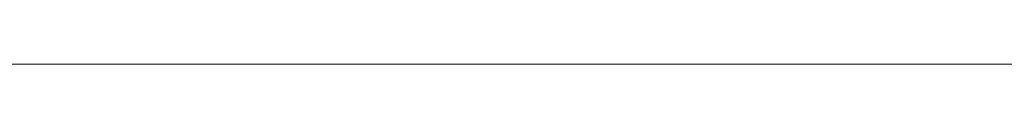
# Model space of a CAD drawing. Units: inches. Extents: x 459864 to 460310, y 324185 to 324787.
# Tile 92 of 112: x 460247.2473 to 460247.3904, y 324283.4832 to 324283.4832. Entities that reach past the tile are written whole.
import ezdxf

# ---------------------------------------------------------------- set-up
doc = ezdxf.new("R2010")
doc.units = ezdxf.units.IN
for name, color, linetype, lineweight in [('A-ANNO-DIMS', 2, 'Continuous', 18), ('L-HRDS', 9, 'Continuous', 18), ('L-SITE-PATT', 252, 'Continuous', 13)]:
    doc.layers.add(name, color=color, linetype=linetype, lineweight=lineweight)
doc.styles.get("Standard").update_dxf_attribs({"font": 'arial.ttf'})
doc.dimstyles.new('ISO-25', dxfattribs={"dimtxt": 6, "dimasz": 2.5, "dimexe": 1.25, "dimexo": 0.625, "dimtad": 1, "dimdec": 1, "dimlunit": 3, "dimtxsty": 'Standard', "dimcen": 2.5, "dimadec": 0, "dimazin": 0, "dimtfac": 1, "dimtdec": 1, "dimtmove": 0, "dimatfit": 3, "dimfxl": 1, "dimarcsym": 0})

# ---------------------------------------------------------------- blocks, each defined once
blk = doc.blocks.new('*D21')
at = {"layer": 'A-ANNO-DIMS', "color": 0, "lineweight": -2, "transparency": 16777216}
for p, q in [((460247.73993, 324715.48323), (460309.58037, 324715.48323)), ((460308.33037, 324712.98323), (460308.33037, 324285.98323)), ((460247.73993, 324283.48323), (460309.58037, 324283.48323))]:
    blk.add_line(p, q, dxfattribs=at)
at = {"layer": 'A-ANNO-DIMS', "color": 0, "transparency": 16777216}
for points in [[(460307.9137, 324712.98323), (460308.74704, 324712.98323), (460308.33037, 324715.48323)], [(460307.9137, 324285.98323), (460308.74704, 324285.98323), (460308.33037, 324283.48323)]]:
    blk.add_solid(points, dxfattribs=at)
at = {"layer": 'Defpoints', "color": 0, "transparency": 16777216}
for p in [(460247.11493, 324715.48323), (460247.11493, 324283.48323), (460308.33037, 324283.48323)]:
    blk.add_point(p, dxfattribs=at)
at = {"layer": 'A-ANNO-DIMS', "color": 0, "transparency": 16777216, "insert": (460304.63988, 324499.48323), "char_height": 6, "attachment_point": 5, "rotation": 90}
blk.add_mtext("36'", dxfattribs=at)

msp = doc.modelspace()

# ---------------------------------------------------------------- hatches: boundary and pattern name
at = {"layer": 'L-SITE-PATT'}
h = msp.add_hatch(dxfattribs=at)
h.set_pattern_fill('DOTS', color=256)
h.paths.add_polyline_path([(460269.80361, 324283.48323), (460247.11493, 324283.48323), (460121.92928, 324283.48323), (460121.92928, 324252.47302), (460117.42928, 324252.47302), (460110.12356, 324252.47302), (460110.12356, 324243.28654), (460080.82954, 324243.28654), (460080.82954, 324252.47302), (460061.11493, 324252.47302), (460061.11493, 324251.88242), (460077.9089, 324251.88242), (460077.9089, 324199.48323), (460080.82954, 324199.48323), (460080.82954, 324207.55322), (460110.12356, 324207.55322), (460110.12356, 324199.48323), (460110.81335, 324199.48323), (460262.11493, 324199.48323), (460269.80361, 324199.48323)], flags=17)
edge = h.paths.add_edge_path(flags=0)
edge.add_ellipse((460222.5903, 324263.81323), major_axis=(-8.48528, 8.48528), ratio=1, start_angle=405, end_angle=495, ccw=False)
edge.add_line((460214.82087, 324254.65989), (460214.83162, 324254.66592))
edge.add_ellipse((460222.5903, 324263.81323), major_axis=(-8.48528, 8.48528), ratio=1, start_angle=405, end_angle=495, ccw=False)
edge.add_line((460210.75891, 324261.78055), (460210.76758, 324261.78682))
edge.add_ellipse((460222.5903, 324263.81323), major_axis=(-8.48528, 8.48528), ratio=1, start_angle=405, end_angle=495, ccw=False)
edge.add_ellipse((460222.5903, 324263.81323), major_axis=(-8.48528, 8.48528), ratio=1, start_angle=392.754016, end_angle=405, ccw=False)
edge.add_ellipse((460222.5903, 324263.81323), major_axis=(-8.48528, 8.48528), ratio=1, start_angle=380.934718, end_angle=392.754016, ccw=False)
edge.add_line((460211.33706, 324267.98503), (460211.3404, 324267.98503))
edge.add_ellipse((460222.5903, 324263.81323), major_axis=(-8.48528, 8.48528), ratio=1, start_angle=380.934718, end_angle=392.754016, ccw=False)
edge.add_ellipse((460222.5903, 324263.81323), major_axis=(-8.48528, 8.48528), ratio=1, start_angle=347.901521, end_angle=380.934718, ccw=False)
edge.add_ellipse((460222.5903, 324263.81323), major_axis=(-8.48528, 8.48528), ratio=1, start_angle=327.061924, end_angle=347.901521, ccw=False)
edge.add_ellipse((460222.5903, 324263.81323), major_axis=(-8.48528, 8.48528), ratio=1, start_angle=278.324642, end_angle=327.061924, ccw=False)
edge.add_line((460225.15828, 324275.53599), (460225.1577, 324275.53464))
edge.add_ellipse((460222.5903, 324263.81323), major_axis=(-8.48528, 8.48528), ratio=1, start_angle=278.324642, end_angle=327.061924, ccw=False)
edge.add_ellipse((460222.5903, 324263.81323), major_axis=(-8.48528, 8.48528), ratio=1, start_angle=260.643569, end_angle=278.324642, ccw=False)
edge.add_ellipse((460222.5903, 324263.81323), major_axis=(-8.48528, 8.48528), ratio=1, start_angle=225, end_angle=260.643569, ccw=False)
edge.add_line((460234.50879, 324265.2428), (460234.50146, 324265.23944))
edge.add_ellipse((460222.5903, 324263.81323), major_axis=(-8.48528, 8.48528), ratio=1, start_angle=225, end_angle=260.643569, ccw=False)
edge.add_ellipse((460222.5903, 324263.81323), major_axis=(-8.48528, 8.48528), ratio=1, start_angle=495, end_angle=585, ccw=False)
edge.add_line((460234.43667, 324261.86121), (460234.42378, 324261.85782))
edge.add_ellipse((460222.5903, 324263.81323), major_axis=(-8.48528, 8.48528), ratio=1, start_angle=495, end_angle=585, ccw=False)
edge.add_line((460227.95013, 324253.06719), (460227.94641, 324253.08314))
edge.add_ellipse((460222.5903, 324263.81323), major_axis=(-8.48528, 8.48528), ratio=1, start_angle=495, end_angle=585, ccw=False)
edge.add_line((460226.22298, 324252.36927), (460226.21103, 324252.37955))
edge.add_ellipse((460222.5903, 324263.81323), major_axis=(-8.48528, 8.48528), ratio=1, start_angle=495, end_angle=585, ccw=False)
h.paths.add_polyline_path([(460219.65145, 324254.34665), (460218.46131, 324253.54498), (460218.27544, 324254.78932), (460219.6424, 324256.54177), (460219.62463, 324260.84756), (460216.11009, 324257.33302), (460214.34997, 324256.97807), (460215.41637, 324259.35568), (460212.52393, 324258.49582), (460213.13731, 324259.9298), (460218.50721, 324263.81323), (460222.5903, 324263.81323), (460222.5903, 324267.8067), (460218.17554, 324272.21231), (460219.02597, 324274.63898), (460222.5903, 324272.81113), (460222.5903, 324275.42332), (460223.0571, 324274.82493), (460222.67523, 324273.49221), (460225.91168, 324267.13461), (460219.62463, 324260.84756)], flags=0)
edge = h.paths.add_edge_path(flags=0)
edge.add_ellipse((460194.57576, 324264.04649), major_axis=(-8.48528, 8.48528), ratio=1, start_angle=495, end_angle=585, ccw=False)
edge.add_line((460199.93559, 324253.30046), (460199.93188, 324253.31641))
edge.add_ellipse((460194.57576, 324264.04649), major_axis=(-8.48528, 8.48528), ratio=1, start_angle=495, end_angle=585, ccw=False)
edge.add_line((460198.20844, 324252.60253), (460198.19649, 324252.61282))
edge.add_ellipse((460194.57576, 324264.04649), major_axis=(-8.48528, 8.48528), ratio=1, start_angle=495, end_angle=585, ccw=False)
edge.add_ellipse((460194.57576, 324264.04649), major_axis=(-8.48528, 8.48528), ratio=1, start_angle=405, end_angle=495, ccw=False)
edge.add_line((460186.80633, 324254.89316), (460186.81708, 324254.89919))
edge.add_ellipse((460194.57576, 324264.04649), major_axis=(-8.48528, 8.48528), ratio=1, start_angle=405, end_angle=495, ccw=False)
edge.add_line((460182.74437, 324262.01382), (460182.75305, 324262.02009))
edge.add_ellipse((460194.57576, 324264.04649), major_axis=(-8.48528, 8.48528), ratio=1, start_angle=405, end_angle=495, ccw=False)
edge.add_ellipse((460194.57576, 324264.04649), major_axis=(-8.48528, 8.48528), ratio=1, start_angle=392.754016, end_angle=405, ccw=False)
edge.add_ellipse((460194.57576, 324264.04649), major_axis=(-8.48528, 8.48528), ratio=1, start_angle=380.934718, end_angle=392.754016, ccw=False)
edge.add_line((460183.32252, 324268.21829), (460183.32587, 324268.21829))
edge.add_ellipse((460194.57576, 324264.04649), major_axis=(-8.48528, 8.48528), ratio=1, start_angle=380.934718, end_angle=392.754016, ccw=False)
edge.add_ellipse((460194.57576, 324264.04649), major_axis=(-8.48528, 8.48528), ratio=1, start_angle=347.901521, end_angle=380.934718, ccw=False)
edge.add_ellipse((460194.57576, 324264.04649), major_axis=(-8.48528, 8.48528), ratio=1, start_angle=327.061924, end_angle=347.901521, ccw=False)
edge.add_ellipse((460194.57576, 324264.04649), major_axis=(-8.48528, 8.48528), ratio=1, start_angle=278.324642, end_angle=327.061924, ccw=False)
edge.add_line((460197.14374, 324275.76926), (460197.14316, 324275.7679))
edge.add_ellipse((460194.57576, 324264.04649), major_axis=(-8.48528, 8.48528), ratio=1, start_angle=278.324642, end_angle=327.061924, ccw=False)
edge.add_ellipse((460194.57576, 324264.04649), major_axis=(-8.48528, 8.48528), ratio=1, start_angle=260.643569, end_angle=278.324642, ccw=False)
edge.add_ellipse((460194.57576, 324264.04649), major_axis=(-8.48528, 8.48528), ratio=1, start_angle=225, end_angle=260.643569, ccw=False)
edge.add_line((460206.49425, 324265.47606), (460206.48692, 324265.47271))
edge.add_ellipse((460194.57576, 324264.04649), major_axis=(-8.48528, 8.48528), ratio=1, start_angle=225, end_angle=260.643569, ccw=False)
edge.add_ellipse((460194.57576, 324264.04649), major_axis=(-8.48528, 8.48528), ratio=1, start_angle=495, end_angle=585, ccw=False)
edge.add_line((460206.42213, 324262.09448), (460206.40925, 324262.09109))
h.paths.add_polyline_path([(460191.61009, 324261.08083), (460191.63691, 324254.57992), (460190.44677, 324253.77825), (460190.2609, 324255.02259), (460191.62786, 324256.77503), (460191.61009, 324261.08083), (460188.09555, 324257.56629), (460186.33543, 324257.21133), (460187.40183, 324259.58894), (460184.5094, 324258.72909), (460185.12278, 324260.16306), (460190.49267, 324264.04649), (460194.57576, 324264.04649), (460194.57576, 324268.03996), (460190.161, 324272.44558), (460191.01143, 324274.87225), (460194.57576, 324273.04439), (460194.57576, 324275.65659), (460195.04256, 324275.0582), (460194.66069, 324273.72548), (460197.89714, 324267.36788)], flags=0)
edge = h.paths.add_edge_path(flags=0)
edge.add_ellipse((460252.91196, 324263.57762), major_axis=(-8.48528, 8.48528), ratio=1, start_angle=405, end_angle=495, ccw=False)
edge.add_line((460241.08058, 324261.54494), (460241.08925, 324261.55121))
edge.add_ellipse((460252.91196, 324263.57762), major_axis=(-8.48528, 8.48528), ratio=1, start_angle=405, end_angle=495, ccw=False)
edge.add_ellipse((460252.91196, 324263.57762), major_axis=(-8.48528, 8.48528), ratio=1, start_angle=392.754016, end_angle=405, ccw=False)
edge.add_ellipse((460252.91196, 324263.57762), major_axis=(-8.48528, 8.48528), ratio=1, start_angle=380.934718, end_angle=392.754016, ccw=False)
edge.add_line((460241.65872, 324267.74942), (460241.66207, 324267.74942))
edge.add_ellipse((460252.91196, 324263.57762), major_axis=(-8.48528, 8.48528), ratio=1, start_angle=380.934718, end_angle=392.754016, ccw=False)
edge.add_ellipse((460252.91196, 324263.57762), major_axis=(-8.48528, 8.48528), ratio=1, start_angle=347.901521, end_angle=380.934718, ccw=False)
edge.add_ellipse((460252.91196, 324263.57762), major_axis=(-8.48528, 8.48528), ratio=1, start_angle=327.061924, end_angle=347.901521, ccw=False)
edge.add_ellipse((460252.91196, 324263.57762), major_axis=(-8.48528, 8.48528), ratio=1, start_angle=278.324642, end_angle=327.061924, ccw=False)
edge.add_line((460255.47994, 324275.30038), (460255.47936, 324275.29902))
edge.add_ellipse((460252.91196, 324263.57762), major_axis=(-8.48528, 8.48528), ratio=1, start_angle=278.324642, end_angle=327.061924, ccw=False)
edge.add_ellipse((460252.91196, 324263.57762), major_axis=(-8.48528, 8.48528), ratio=1, start_angle=260.643569, end_angle=278.324642, ccw=False)
edge.add_ellipse((460252.91196, 324263.57762), major_axis=(-8.48528, 8.48528), ratio=1, start_angle=225, end_angle=260.643569, ccw=False)
edge.add_line((460264.83046, 324265.00718), (460264.82312, 324265.00383))
edge.add_ellipse((460252.91196, 324263.57762), major_axis=(-8.48528, 8.48528), ratio=1, start_angle=225, end_angle=260.643569, ccw=False)
edge.add_ellipse((460252.91196, 324263.57762), major_axis=(-8.48528, 8.48528), ratio=1, start_angle=495, end_angle=585, ccw=False)
edge.add_line((460264.75833, 324261.6256), (460264.74545, 324261.62221))
edge.add_ellipse((460252.91196, 324263.57762), major_axis=(-8.48528, 8.48528), ratio=1, start_angle=495, end_angle=585, ccw=False)
edge.add_line((460258.2718, 324252.83158), (460258.26808, 324252.84753))
edge.add_ellipse((460252.91196, 324263.57762), major_axis=(-8.48528, 8.48528), ratio=1, start_angle=495, end_angle=585, ccw=False)
edge.add_line((460256.54464, 324252.13365), (460256.5327, 324252.14394))
edge.add_ellipse((460252.91196, 324263.57762), major_axis=(-8.48528, 8.48528), ratio=1, start_angle=495, end_angle=585, ccw=False)
edge.add_ellipse((460252.91196, 324263.57762), major_axis=(-8.48528, 8.48528), ratio=1, start_angle=405, end_angle=495, ccw=False)
edge.add_line((460245.14253, 324254.42428), (460245.15329, 324254.43031))
h.paths.add_polyline_path([(460244.67163, 324256.74245), (460245.73803, 324259.12007), (460242.8456, 324258.26021), (460243.45898, 324259.69418), (460248.82888, 324263.57762), (460252.91196, 324263.57762), (460252.91196, 324267.57108), (460248.4972, 324271.9767), (460249.34763, 324274.40337), (460252.91196, 324272.57552), (460252.91196, 324275.18771), (460253.37876, 324274.58932), (460252.9969, 324273.2566), (460256.23334, 324266.899), (460249.9463, 324260.61195), (460249.97312, 324254.11104), (460248.78298, 324253.30937), (460248.5971, 324254.55371), (460249.96406, 324256.30615), (460249.9463, 324260.61195), (460246.43175, 324257.09741)], flags=0)
edge = h.paths.add_edge_path(flags=0)
edge.add_ellipse((460167.43869, 324262.83279), major_axis=(-8.48528, 8.48528), ratio=1, start_angle=495, end_angle=585, ccw=False)
edge.add_line((460172.79852, 324252.08676), (460172.79481, 324252.1027))
edge.add_ellipse((460167.43869, 324262.83279), major_axis=(-8.48528, 8.48528), ratio=1, start_angle=495, end_angle=585, ccw=False)
edge.add_line((460171.07137, 324251.38883), (460171.05942, 324251.39911))
edge.add_ellipse((460167.43869, 324262.83279), major_axis=(-8.48528, 8.48528), ratio=1, start_angle=495, end_angle=585, ccw=False)
edge.add_ellipse((460167.43869, 324262.83279), major_axis=(-8.48528, 8.48528), ratio=1, start_angle=405, end_angle=495, ccw=False)
edge.add_line((460159.66926, 324253.67945), (460159.68001, 324253.68548))
edge.add_ellipse((460167.43869, 324262.83279), major_axis=(-8.48528, 8.48528), ratio=1, start_angle=405, end_angle=495, ccw=False)
edge.add_line((460155.6073, 324260.80011), (460155.61598, 324260.80639))
edge.add_ellipse((460167.43869, 324262.83279), major_axis=(-8.48528, 8.48528), ratio=1, start_angle=405, end_angle=495, ccw=False)
edge.add_ellipse((460167.43869, 324262.83279), major_axis=(-8.48528, 8.48528), ratio=1, start_angle=392.754016, end_angle=405, ccw=False)
edge.add_ellipse((460167.43869, 324262.83279), major_axis=(-8.48528, 8.48528), ratio=1, start_angle=380.934718, end_angle=392.754016, ccw=False)
edge.add_line((460156.18545, 324267.00459), (460156.1888, 324267.00459))
edge.add_ellipse((460167.43869, 324262.83279), major_axis=(-8.48528, 8.48528), ratio=1, start_angle=380.934718, end_angle=392.754016, ccw=False)
edge.add_ellipse((460167.43869, 324262.83279), major_axis=(-8.48528, 8.48528), ratio=1, start_angle=347.901521, end_angle=380.934718, ccw=False)
edge.add_ellipse((460167.43869, 324262.83279), major_axis=(-8.48528, 8.48528), ratio=1, start_angle=327.061924, end_angle=347.901521, ccw=False)
edge.add_ellipse((460167.43869, 324262.83279), major_axis=(-8.48528, 8.48528), ratio=1, start_angle=278.324642, end_angle=327.061924, ccw=False)
edge.add_line((460170.00667, 324274.55555), (460170.00609, 324274.5542))
edge.add_ellipse((460167.43869, 324262.83279), major_axis=(-8.48528, 8.48528), ratio=1, start_angle=278.324642, end_angle=327.061924, ccw=False)
edge.add_ellipse((460167.43869, 324262.83279), major_axis=(-8.48528, 8.48528), ratio=1, start_angle=260.643569, end_angle=278.324642, ccw=False)
edge.add_ellipse((460167.43869, 324262.83279), major_axis=(-8.48528, 8.48528), ratio=1, start_angle=225, end_angle=260.643569, ccw=False)
edge.add_line((460179.35719, 324264.26236), (460179.34985, 324264.259))
edge.add_ellipse((460167.43869, 324262.83279), major_axis=(-8.48528, 8.48528), ratio=1, start_angle=225, end_angle=260.643569, ccw=False)
edge.add_ellipse((460167.43869, 324262.83279), major_axis=(-8.48528, 8.48528), ratio=1, start_angle=495, end_angle=585, ccw=False)
edge.add_line((460179.28506, 324260.88078), (460179.27218, 324260.87738))
h.paths.add_polyline_path([(460164.47302, 324259.86713), (460164.49985, 324253.36622), (460163.30971, 324252.56455), (460163.12383, 324253.80888), (460164.49079, 324255.56133), (460164.47302, 324259.86713), (460160.95848, 324256.35258), (460159.19836, 324255.99763), (460160.26476, 324258.37524), (460157.37233, 324257.51539), (460157.98571, 324258.94936), (460163.35561, 324262.83279), (460167.43869, 324262.83279), (460167.43869, 324266.82626), (460163.02393, 324271.23187), (460163.87436, 324273.65854), (460167.43869, 324271.83069), (460167.43869, 324274.44288), (460167.90549, 324273.84449), (460167.52362, 324272.51177), (460170.76007, 324266.15417)], flags=0)
edge = h.paths.add_edge_path(flags=0)
edge.add_ellipse((460140.75809, 324262.36958), major_axis=(-8.48528, 8.48528), ratio=1, start_angle=495, end_angle=585, ccw=False)
edge.add_line((460146.11792, 324251.62355), (460146.11421, 324251.6395))
edge.add_ellipse((460140.75809, 324262.36958), major_axis=(-8.48528, 8.48528), ratio=1, start_angle=495, end_angle=585, ccw=False)
edge.add_line((460144.39077, 324250.92562), (460144.37882, 324250.93591))
edge.add_ellipse((460140.75809, 324262.36958), major_axis=(-8.48528, 8.48528), ratio=1, start_angle=495, end_angle=585, ccw=False)
edge.add_ellipse((460140.75809, 324262.36958), major_axis=(-8.48528, 8.48528), ratio=1, start_angle=405, end_angle=495, ccw=False)
edge.add_line((460132.98866, 324253.21625), (460132.99941, 324253.22228))
edge.add_ellipse((460140.75809, 324262.36958), major_axis=(-8.48528, 8.48528), ratio=1, start_angle=405, end_angle=495, ccw=False)
edge.add_line((460128.9267, 324260.33691), (460128.93538, 324260.34318))
edge.add_ellipse((460140.75809, 324262.36958), major_axis=(-8.48528, 8.48528), ratio=1, start_angle=405, end_angle=495, ccw=False)
edge.add_ellipse((460140.75809, 324262.36958), major_axis=(-8.48528, 8.48528), ratio=1, start_angle=392.754016, end_angle=405, ccw=False)
edge.add_ellipse((460140.75809, 324262.36958), major_axis=(-8.48528, 8.48528), ratio=1, start_angle=380.934718, end_angle=392.754016, ccw=False)
edge.add_line((460129.50485, 324266.54138), (460129.5082, 324266.54138))
edge.add_ellipse((460140.75809, 324262.36958), major_axis=(-8.48528, 8.48528), ratio=1, start_angle=380.934718, end_angle=392.754016, ccw=False)
edge.add_ellipse((460140.75809, 324262.36958), major_axis=(-8.48528, 8.48528), ratio=1, start_angle=347.901521, end_angle=380.934718, ccw=False)
edge.add_ellipse((460140.75809, 324262.36958), major_axis=(-8.48528, 8.48528), ratio=1, start_angle=327.061924, end_angle=347.901521, ccw=False)
edge.add_ellipse((460140.75809, 324262.36958), major_axis=(-8.48528, 8.48528), ratio=1, start_angle=278.324642, end_angle=327.061924, ccw=False)
edge.add_line((460143.32607, 324274.09235), (460143.32549, 324274.09099))
edge.add_ellipse((460140.75809, 324262.36958), major_axis=(-8.48528, 8.48528), ratio=1, start_angle=278.324642, end_angle=327.061924, ccw=False)
edge.add_ellipse((460140.75809, 324262.36958), major_axis=(-8.48528, 8.48528), ratio=1, start_angle=260.643569, end_angle=278.324642, ccw=False)
edge.add_ellipse((460140.75809, 324262.36958), major_axis=(-8.48528, 8.48528), ratio=1, start_angle=225, end_angle=260.643569, ccw=False)
edge.add_line((460152.67658, 324263.79915), (460152.66925, 324263.7958))
edge.add_ellipse((460140.75809, 324262.36958), major_axis=(-8.48528, 8.48528), ratio=1, start_angle=225, end_angle=260.643569, ccw=False)
edge.add_ellipse((460140.75809, 324262.36958), major_axis=(-8.48528, 8.48528), ratio=1, start_angle=495, end_angle=585, ccw=False)
edge.add_line((460152.60446, 324260.41757), (460152.59158, 324260.41418))
h.paths.add_polyline_path([(460137.79242, 324259.40392), (460137.81925, 324252.90301), (460136.6291, 324252.10134), (460136.44323, 324253.34568), (460137.81019, 324255.09812), (460137.79242, 324259.40392), (460134.27788, 324255.88938), (460132.51776, 324255.53442), (460133.58416, 324257.91203), (460130.69173, 324257.05218), (460131.30511, 324258.48615), (460136.675, 324262.36958), (460140.75809, 324262.36958), (460140.75809, 324266.36305), (460136.34333, 324270.76867), (460137.19376, 324273.19534), (460140.75809, 324271.36749), (460140.75809, 324273.97968), (460141.22489, 324273.38129), (460140.84302, 324272.04857), (460144.07947, 324265.69097)], flags=0)
h.paths.add_polyline_path([(460110.12356, 324227.41387), (460080.82954, 324227.41387), (460080.82954, 324235.48385), (460110.12356, 324235.48385)], flags=16)
h.paths.add_polyline_path([(460110.12356, 324220.79663), (460110.12356, 324212.72665), (460080.82954, 324212.72665), (460080.82954, 324220.79663)], flags=16)
h.paths.add_polyline_path([(460269.80361, 324283.48323), (460247.11493, 324283.48323), (460121.92928, 324283.48323), (460121.92928, 324252.47302), (460117.42928, 324252.47302), (460110.12356, 324252.47302), (460110.12356, 324243.28654), (460080.82954, 324243.28654), (460080.82954, 324252.47302), (460061.11493, 324252.47302), (460061.11493, 324251.88242), (460077.9089, 324251.88242), (460077.9089, 324199.48323), (460080.82954, 324199.48323), (460080.82954, 324207.55322), (460110.12356, 324207.55322), (460110.12356, 324199.48323), (460262.11493, 324199.48323), (460269.80361, 324199.48323)], flags=17)
h.paths.add_polyline_path([(460219.65145, 324254.34665), (460218.46131, 324253.54498), (460218.27544, 324254.78932), (460219.6424, 324256.54177), (460219.62463, 324260.84756), (460216.11009, 324257.33302), (460214.34997, 324256.97807), (460215.41637, 324259.35568), (460212.52393, 324258.49582), (460213.13731, 324259.9298), (460218.50721, 324263.81323), (460222.5903, 324263.81323), (460220.18049, 324266.22304), (460215.46096, 324265.30765), (460211.83453, 324266.13655), (460216.24662, 324267.98503), (460218.4185, 324267.98503), (460222.5903, 324263.81323), (460222.5903, 324267.8067), (460218.17554, 324272.21231), (460219.02597, 324274.63898), (460222.5903, 324272.81113), (460222.5903, 324275.42332), (460223.0571, 324274.82493), (460222.67523, 324273.49221), (460225.91168, 324267.13461), (460222.5903, 324263.81323), (460231.38287, 324263.81323), (460228.48472, 324262.48783), (460224.42521, 324261.97832), (460228.6799, 324257.72362), (460228.96584, 324254.79101), (460227.14177, 324256.53663), (460227.54207, 324254.81857), (460227.33334, 324253.61447), (460222.5903, 324259.98463), (460222.5903, 324255.49667), (460221.37741, 324256.54085), (460220.57579, 324261.79873), (460219.62463, 324260.84756)], flags=0)
h.paths.add_polyline_path([(460199.12723, 324256.7699), (460199.52753, 324255.05184), (460199.31881, 324253.84773), (460194.57576, 324260.21789), (460194.57576, 324255.72993), (460193.36287, 324256.77411), (460192.56126, 324262.03199), (460191.61009, 324261.08083), (460191.63691, 324254.57992), (460190.44677, 324253.77825), (460190.2609, 324255.02259), (460191.62786, 324256.77503), (460191.61009, 324261.08083), (460188.09555, 324257.56629), (460186.33543, 324257.21133), (460187.40183, 324259.58894), (460184.5094, 324258.72909), (460185.12278, 324260.16306), (460190.49267, 324264.04649), (460194.57576, 324264.04649), (460192.16595, 324266.4563), (460187.44642, 324265.54091), (460183.82, 324266.36982), (460188.23208, 324268.21829), (460190.40396, 324268.21829), (460194.57576, 324264.04649), (460194.57576, 324268.03996), (460190.161, 324272.44558), (460191.01143, 324274.87225), (460194.57576, 324273.04439), (460194.57576, 324275.65659), (460195.04256, 324275.0582), (460194.66069, 324273.72548), (460197.89714, 324267.36788), (460194.57576, 324264.04649), (460203.36833, 324264.04649), (460200.47018, 324262.72109), (460196.41067, 324262.21158), (460200.66536, 324257.95689), (460200.9513, 324255.02428)], flags=0)
h.paths.add_polyline_path([(460244.67163, 324256.74245), (460245.73803, 324259.12007), (460242.8456, 324258.26021), (460243.45898, 324259.69418), (460248.82888, 324263.57762), (460252.91196, 324263.57762), (460250.50215, 324265.98742), (460245.78262, 324265.07203), (460242.1562, 324265.90094), (460246.56828, 324267.74942), (460248.74016, 324267.74942), (460252.91196, 324263.57762), (460252.91196, 324267.57108), (460248.4972, 324271.9767), (460249.34763, 324274.40337), (460252.91196, 324272.57552), (460252.91196, 324275.18771), (460253.37876, 324274.58932), (460252.9969, 324273.2566), (460256.23334, 324266.899), (460252.91196, 324263.57762), (460261.70454, 324263.57762), (460258.80638, 324262.25221), (460254.74687, 324261.7427), (460259.00157, 324257.48801), (460259.2875, 324254.5554), (460257.46343, 324256.30102), (460257.86373, 324254.58296), (460257.65501, 324253.37885), (460252.91196, 324259.74901), (460252.91196, 324255.26105), (460251.69907, 324256.30524), (460250.89746, 324261.56311), (460249.9463, 324260.61195), (460249.97312, 324254.11104), (460248.78298, 324253.30937), (460248.5971, 324254.55371), (460249.96406, 324256.30615), (460249.9463, 324260.61195), (460246.43175, 324257.09741)], flags=0)
h.paths.add_polyline_path([(460173.52829, 324256.74319), (460173.81423, 324253.81058), (460171.99016, 324255.55619), (460172.39046, 324253.83814), (460172.18174, 324252.63403), (460167.43869, 324259.00419), (460167.43869, 324254.51623), (460166.2258, 324255.56041), (460165.42419, 324260.81829), (460164.47302, 324259.86713), (460164.49985, 324253.36622), (460163.30971, 324252.56455), (460163.12383, 324253.80888), (460164.49079, 324255.56133), (460164.47302, 324259.86713), (460160.95848, 324256.35258), (460159.19836, 324255.99763), (460160.26476, 324258.37524), (460157.37233, 324257.51539), (460157.98571, 324258.94936), (460163.35561, 324262.83279), (460167.43869, 324262.83279), (460165.02888, 324265.2426), (460160.30935, 324264.32721), (460156.68293, 324265.15611), (460161.09501, 324267.00459), (460163.26689, 324267.00459), (460167.43869, 324262.83279), (460167.43869, 324266.82626), (460163.02393, 324271.23187), (460163.87436, 324273.65854), (460167.43869, 324271.83069), (460167.43869, 324274.44288), (460167.90549, 324273.84449), (460167.52362, 324272.51177), (460170.76007, 324266.15417), (460167.43869, 324262.83279), (460176.23127, 324262.83279), (460173.33311, 324261.50739), (460169.2736, 324260.99788)], flags=0)
h.paths.add_polyline_path([(460146.84769, 324256.27998), (460147.13363, 324253.34737), (460145.30956, 324255.09299), (460145.70986, 324253.37493), (460145.50114, 324252.17082), (460140.75809, 324258.54098), (460140.75809, 324254.05302), (460139.5452, 324255.0972), (460138.74359, 324260.35508), (460137.79242, 324259.40392), (460137.81925, 324252.90301), (460136.6291, 324252.10134), (460136.44323, 324253.34568), (460137.81019, 324255.09812), (460137.79242, 324259.40392), (460134.27788, 324255.88938), (460132.51776, 324255.53442), (460133.58416, 324257.91203), (460130.69173, 324257.05218), (460131.30511, 324258.48615), (460136.675, 324262.36958), (460140.75809, 324262.36958), (460138.34828, 324264.77939), (460133.62875, 324263.864), (460130.00233, 324264.69291), (460134.41441, 324266.54138), (460136.58629, 324266.54138), (460140.75809, 324262.36958), (460140.75809, 324266.36305), (460136.34333, 324270.76867), (460137.19376, 324273.19534), (460140.75809, 324271.36749), (460140.75809, 324273.97968), (460141.22489, 324273.38129), (460140.84302, 324272.04857), (460144.07947, 324265.69097), (460140.75809, 324262.36958), (460149.55066, 324262.36958), (460146.65251, 324261.04418), (460142.593, 324260.53467)], flags=0)
edge = h.paths.add_edge_path()
edge.add_line((460269.80361, 324272.54905), (460260.88148, 324272.54905))
edge.add_ellipse((460252.91196, 324263.57762), major_axis=(-8.48528, 8.48528), ratio=1, start_angle=260.643569, end_angle=273.384624, ccw=False)
edge.add_line((460262.28261, 324271.09211), (460262.26055, 324271.09106))
edge.add_ellipse((460252.91196, 324263.57762), major_axis=(-8.48528, 8.48528), ratio=1, start_angle=260.643569, end_angle=273.384624, ccw=False)
edge.add_ellipse((460252.91196, 324263.57762), major_axis=(-8.48528, 8.48528), ratio=1, start_angle=225, end_angle=260.643569, ccw=False)
edge.add_line((460263.60857, 324269.06329), (460263.57165, 324269.05828))
edge.add_ellipse((460252.91196, 324263.57762), major_axis=(-8.48528, 8.48528), ratio=1, start_angle=225, end_angle=260.643569, ccw=False)
edge.add_line((460264.61546, 324266.30554), (460264.58536, 324266.3052))
edge.add_ellipse((460252.91196, 324263.57762), major_axis=(-8.48528, 8.48528), ratio=1, start_angle=225, end_angle=260.643569, ccw=False)
edge.add_line((460264.83046, 324265.00718), (460264.82312, 324265.00383))
edge.add_ellipse((460252.91196, 324263.57762), major_axis=(-8.48528, 8.48528), ratio=1, start_angle=225, end_angle=260.643569, ccw=False)
edge.add_ellipse((460252.91196, 324263.57762), major_axis=(-8.48528, 8.48528), ratio=1, start_angle=495, end_angle=585, ccw=False)
edge.add_line((460264.75833, 324261.6256), (460264.74545, 324261.62221))
edge.add_ellipse((460252.91196, 324263.57762), major_axis=(-8.48528, 8.48528), ratio=1, start_angle=495, end_angle=585, ccw=False)
edge.add_line((460263.4422, 324257.73902), (460263.38926, 324257.77924))
edge.add_ellipse((460252.91196, 324263.57762), major_axis=(-8.48528, 8.48528), ratio=1, start_angle=495, end_angle=585, ccw=False)
edge.add_line((460258.12807, 324252.7435), (460258.10188, 324252.77868))
edge.add_ellipse((460252.91196, 324263.57762), major_axis=(-8.48528, 8.48528), ratio=1, start_angle=495, end_angle=585, ccw=False)
edge.add_line((460256.54464, 324252.13365), (460256.5327, 324252.14394))
edge.add_ellipse((460252.91196, 324263.57762), major_axis=(-8.48528, 8.48528), ratio=1, start_angle=495, end_angle=585, ccw=False)
edge.add_ellipse((460252.91196, 324263.57762), major_axis=(-8.48528, 8.48528), ratio=1, start_angle=405, end_angle=495, ccw=False)
edge.add_line((460250.59399, 324251.78041), (460250.60465, 324251.81982))
edge.add_ellipse((460252.91196, 324263.57762), major_axis=(-8.48528, 8.48528), ratio=1, start_angle=405, end_angle=495, ccw=False)
edge.add_line((460245.14253, 324254.42428), (460245.15329, 324254.43031))
edge.add_ellipse((460252.91196, 324263.57762), major_axis=(-8.48528, 8.48528), ratio=1, start_angle=405, end_angle=495, ccw=False)
edge.add_line((460243.52459, 324256.059), (460243.56034, 324256.09136))
edge.add_ellipse((460252.91196, 324263.57762), major_axis=(-8.48528, 8.48528), ratio=1, start_angle=405, end_angle=495, ccw=False)
edge.add_line((460241.4401, 324259.89273), (460241.52244, 324259.89588))
edge.add_ellipse((460252.91196, 324263.57762), major_axis=(-8.48528, 8.48528), ratio=1, start_angle=405, end_angle=495, ccw=False)
edge.add_line((460241.08058, 324261.54494), (460241.08925, 324261.55121))
edge.add_ellipse((460252.91196, 324263.57762), major_axis=(-8.48528, 8.48528), ratio=1, start_angle=405, end_angle=495, ccw=False)
edge.add_ellipse((460252.91196, 324263.57762), major_axis=(-8.48528, 8.48528), ratio=1, start_angle=392.754016, end_angle=405, ccw=False)
edge.add_line((460241.0503, 324265.43761), (460241.06257, 324265.44275))
edge.add_ellipse((460252.91196, 324263.57762), major_axis=(-8.48528, 8.48528), ratio=1, start_angle=392.754016, end_angle=405, ccw=False)
edge.add_ellipse((460252.91196, 324263.57762), major_axis=(-8.48528, 8.48528), ratio=1, start_angle=380.934718, end_angle=392.754016, ccw=False)
edge.add_line((460241.45189, 324267.17639), (460241.46904, 324267.17099))
edge.add_ellipse((460252.91196, 324263.57762), major_axis=(-8.48528, 8.48528), ratio=1, start_angle=380.934718, end_angle=392.754016, ccw=False)
edge.add_line((460241.65872, 324267.74942), (460241.66207, 324267.74942))
edge.add_ellipse((460252.91196, 324263.57762), major_axis=(-8.48528, 8.48528), ratio=1, start_angle=380.934718, end_angle=392.754016, ccw=False)
edge.add_ellipse((460252.91196, 324263.57762), major_axis=(-8.48528, 8.48528), ratio=1, start_angle=356.615376, end_angle=380.934718, ccw=False)
edge.add_line((460244.88029, 324272.48765), (460244.71265, 324272.54905))
edge.add_line((460244.71265, 324272.54905), (460230.81741, 324272.54905))
edge.add_ellipse((460222.5903, 324263.81323), major_axis=(-8.48528, 8.48528), ratio=1, start_angle=260.643569, end_angle=271.717775, ccw=False)
edge.add_ellipse((460222.5903, 324263.81323), major_axis=(-8.48528, 8.48528), ratio=1, start_angle=225, end_angle=260.643569, ccw=False)
edge.add_line((460233.2869, 324269.29891), (460233.24999, 324269.2939))
edge.add_ellipse((460222.5903, 324263.81323), major_axis=(-8.48528, 8.48528), ratio=1, start_angle=225, end_angle=260.643569, ccw=False)
edge.add_line((460234.2938, 324266.54115), (460234.26369, 324266.54081))
edge.add_ellipse((460222.5903, 324263.81323), major_axis=(-8.48528, 8.48528), ratio=1, start_angle=225, end_angle=260.643569, ccw=False)
edge.add_line((460234.50879, 324265.2428), (460234.50146, 324265.23944))
edge.add_ellipse((460222.5903, 324263.81323), major_axis=(-8.48528, 8.48528), ratio=1, start_angle=225, end_angle=260.643569, ccw=False)
edge.add_ellipse((460222.5903, 324263.81323), major_axis=(-8.48528, 8.48528), ratio=1, start_angle=495, end_angle=585, ccw=False)
edge.add_line((460234.43667, 324261.86121), (460234.42378, 324261.85782))
edge.add_ellipse((460222.5903, 324263.81323), major_axis=(-8.48528, 8.48528), ratio=1, start_angle=495, end_angle=585, ccw=False)
edge.add_line((460233.12054, 324257.97463), (460233.06759, 324258.01485))
edge.add_ellipse((460222.5903, 324263.81323), major_axis=(-8.48528, 8.48528), ratio=1, start_angle=495, end_angle=585, ccw=False)
edge.add_line((460227.8064, 324252.97912), (460227.78021, 324253.0143))
edge.add_ellipse((460222.5903, 324263.81323), major_axis=(-8.48528, 8.48528), ratio=1, start_angle=495, end_angle=585, ccw=False)
edge.add_line((460226.22298, 324252.36927), (460226.21103, 324252.37955))
edge.add_ellipse((460222.5903, 324263.81323), major_axis=(-8.48528, 8.48528), ratio=1, start_angle=495, end_angle=585, ccw=False)
edge.add_ellipse((460222.5903, 324263.81323), major_axis=(-8.48528, 8.48528), ratio=1, start_angle=405, end_angle=495, ccw=False)
edge.add_line((460220.27232, 324252.01602), (460220.28299, 324252.05543))
edge.add_ellipse((460222.5903, 324263.81323), major_axis=(-8.48528, 8.48528), ratio=1, start_angle=405, end_angle=495, ccw=False)
edge.add_line((460214.82087, 324254.65989), (460214.83162, 324254.66592))
edge.add_ellipse((460222.5903, 324263.81323), major_axis=(-8.48528, 8.48528), ratio=1, start_angle=405, end_angle=495, ccw=False)
edge.add_line((460213.20292, 324256.29462), (460213.23868, 324256.32697))
edge.add_ellipse((460222.5903, 324263.81323), major_axis=(-8.48528, 8.48528), ratio=1, start_angle=405, end_angle=495, ccw=False)
edge.add_line((460211.11844, 324260.12834), (460211.20077, 324260.13149))
edge.add_ellipse((460222.5903, 324263.81323), major_axis=(-8.48528, 8.48528), ratio=1, start_angle=405, end_angle=495, ccw=False)
edge.add_line((460210.75891, 324261.78055), (460210.76758, 324261.78682))
edge.add_ellipse((460222.5903, 324263.81323), major_axis=(-8.48528, 8.48528), ratio=1, start_angle=405, end_angle=495, ccw=False)
edge.add_ellipse((460222.5903, 324263.81323), major_axis=(-8.48528, 8.48528), ratio=1, start_angle=392.754016, end_angle=405, ccw=False)
edge.add_line((460210.72863, 324265.67323), (460210.7409, 324265.67836))
edge.add_ellipse((460222.5903, 324263.81323), major_axis=(-8.48528, 8.48528), ratio=1, start_angle=392.754016, end_angle=405, ccw=False)
edge.add_ellipse((460222.5903, 324263.81323), major_axis=(-8.48528, 8.48528), ratio=1, start_angle=380.934718, end_angle=392.754016, ccw=False)
edge.add_line((460211.13022, 324267.412), (460211.14738, 324267.4066))
edge.add_ellipse((460222.5903, 324263.81323), major_axis=(-8.48528, 8.48528), ratio=1, start_angle=380.934718, end_angle=392.754016, ccw=False)
edge.add_line((460211.33706, 324267.98503), (460211.3404, 324267.98503))
edge.add_ellipse((460222.5903, 324263.81323), major_axis=(-8.48528, 8.48528), ratio=1, start_angle=380.934718, end_angle=392.754016, ccw=False)
edge.add_ellipse((460222.5903, 324263.81323), major_axis=(-8.48528, 8.48528), ratio=1, start_angle=358.282225, end_angle=380.934718, ccw=False)
edge.add_line((460213.70452, 324271.90183), (460213.70904, 324271.86897))
edge.add_ellipse((460222.5903, 324263.81323), major_axis=(-8.48528, 8.48528), ratio=1, start_angle=358.282225, end_angle=380.934718, ccw=False)
edge.add_line((460214.36318, 324272.54905), (460203.07832, 324272.54905))
edge.add_line((460203.07832, 324272.54905), (460203.06034, 324272.53108))
edge.add_ellipse((460194.57576, 324264.04649), major_axis=(-8.48528, 8.48528), ratio=1, start_angle=260.643569, end_angle=270.11679, ccw=False)
edge.add_line((460203.95659, 324271.56147), (460203.92091, 324271.55978))
edge.add_ellipse((460194.57576, 324264.04649), major_axis=(-8.48528, 8.48528), ratio=1, start_angle=260.643569, end_angle=270.11679, ccw=False)
edge.add_ellipse((460194.57576, 324264.04649), major_axis=(-8.48528, 8.48528), ratio=1, start_angle=225, end_angle=260.643569, ccw=False)
edge.add_line((460205.27237, 324269.53217), (460205.23545, 324269.52716))
edge.add_ellipse((460194.57576, 324264.04649), major_axis=(-8.48528, 8.48528), ratio=1, start_angle=225, end_angle=260.643569, ccw=False)
edge.add_line((460206.27926, 324266.77442), (460206.24915, 324266.77407))
edge.add_ellipse((460194.57576, 324264.04649), major_axis=(-8.48528, 8.48528), ratio=1, start_angle=225, end_angle=260.643569, ccw=False)
edge.add_line((460206.49425, 324265.47606), (460206.48692, 324265.47271))
edge.add_ellipse((460194.57576, 324264.04649), major_axis=(-8.48528, 8.48528), ratio=1, start_angle=225, end_angle=260.643569, ccw=False)
edge.add_ellipse((460194.57576, 324264.04649), major_axis=(-8.48528, 8.48528), ratio=1, start_angle=495, end_angle=585, ccw=False)
edge.add_line((460206.42213, 324262.09448), (460206.40925, 324262.09109))
edge.add_ellipse((460194.57576, 324264.04649), major_axis=(-8.48528, 8.48528), ratio=1, start_angle=495, end_angle=585, ccw=False)
edge.add_line((460205.106, 324258.2079), (460205.05306, 324258.24812))
edge.add_ellipse((460194.57576, 324264.04649), major_axis=(-8.48528, 8.48528), ratio=1, start_angle=495, end_angle=585, ccw=False)
edge.add_line((460199.79187, 324253.21238), (460199.76568, 324253.24756))
edge.add_ellipse((460194.57576, 324264.04649), major_axis=(-8.48528, 8.48528), ratio=1, start_angle=495, end_angle=585, ccw=False)
edge.add_line((460198.20844, 324252.60253), (460198.19649, 324252.61282))
edge.add_ellipse((460194.57576, 324264.04649), major_axis=(-8.48528, 8.48528), ratio=1, start_angle=495, end_angle=585, ccw=False)
edge.add_ellipse((460194.57576, 324264.04649), major_axis=(-8.48528, 8.48528), ratio=1, start_angle=405, end_angle=495, ccw=False)
edge.add_line((460192.25779, 324252.24929), (460192.26845, 324252.2887))
edge.add_ellipse((460194.57576, 324264.04649), major_axis=(-8.48528, 8.48528), ratio=1, start_angle=405, end_angle=495, ccw=False)
edge.add_line((460186.80633, 324254.89316), (460186.81708, 324254.89919))
edge.add_ellipse((460194.57576, 324264.04649), major_axis=(-8.48528, 8.48528), ratio=1, start_angle=405, end_angle=495, ccw=False)
edge.add_line((460185.18839, 324256.52788), (460185.22414, 324256.56024))
edge.add_ellipse((460194.57576, 324264.04649), major_axis=(-8.48528, 8.48528), ratio=1, start_angle=405, end_angle=495, ccw=False)
edge.add_line((460183.1039, 324260.3616), (460183.18624, 324260.36476))
edge.add_ellipse((460194.57576, 324264.04649), major_axis=(-8.48528, 8.48528), ratio=1, start_angle=405, end_angle=495, ccw=False)
edge.add_line((460182.74437, 324262.01382), (460182.75305, 324262.02009))
edge.add_ellipse((460194.57576, 324264.04649), major_axis=(-8.48528, 8.48528), ratio=1, start_angle=405, end_angle=495, ccw=False)
edge.add_ellipse((460194.57576, 324264.04649), major_axis=(-8.48528, 8.48528), ratio=1, start_angle=392.754016, end_angle=405, ccw=False)
edge.add_line((460182.7141, 324265.90649), (460182.72636, 324265.91163))
edge.add_ellipse((460194.57576, 324264.04649), major_axis=(-8.48528, 8.48528), ratio=1, start_angle=392.754016, end_angle=405, ccw=False)
edge.add_ellipse((460194.57576, 324264.04649), major_axis=(-8.48528, 8.48528), ratio=1, start_angle=380.934718, end_angle=392.754016, ccw=False)
edge.add_line((460183.11568, 324267.64527), (460183.13284, 324267.63987))
edge.add_ellipse((460194.57576, 324264.04649), major_axis=(-8.48528, 8.48528), ratio=1, start_angle=380.934718, end_angle=392.754016, ccw=False)
edge.add_line((460183.32252, 324268.21829), (460183.32587, 324268.21829))
edge.add_ellipse((460194.57576, 324264.04649), major_axis=(-8.48528, 8.48528), ratio=1, start_angle=380.934718, end_angle=392.754016, ccw=False)
edge.add_ellipse((460194.57576, 324264.04649), major_axis=(-8.48528, 8.48528), ratio=1, start_angle=359.88321, end_angle=380.934718, ccw=False)
edge.add_line((460184.49136, 324270.61077), (460184.55315, 324270.61077))
edge.add_ellipse((460194.57576, 324264.04649), major_axis=(-8.48528, 8.48528), ratio=1, start_angle=359.88321, end_angle=380.934718, ccw=False)
edge.add_line((460185.34584, 324271.76024), (460185.37863, 324271.72802))
edge.add_ellipse((460194.57576, 324264.04649), major_axis=(-8.48528, 8.48528), ratio=1, start_angle=359.88321, end_angle=380.934718, ccw=False)
edge.add_line((460185.69672, 324272.08618), (460185.633, 324272.54905))
edge.add_line((460185.633, 324272.54905), (460174.68345, 324272.54905))
edge.add_line((460174.68345, 324272.54905), (460174.60605, 324272.45718))
edge.add_ellipse((460167.43869, 324262.83279), major_axis=(-8.48528, 8.48528), ratio=1, start_angle=260.643569, end_angle=278.324642, ccw=False)
edge.add_ellipse((460167.43869, 324262.83279), major_axis=(-8.48528, 8.48528), ratio=1, start_angle=225, end_angle=260.643569, ccw=False)
edge.add_line((460178.1353, 324268.31847), (460178.09838, 324268.31346))
edge.add_ellipse((460167.43869, 324262.83279), major_axis=(-8.48528, 8.48528), ratio=1, start_angle=225, end_angle=260.643569, ccw=False)
edge.add_line((460179.14219, 324265.56072), (460179.11209, 324265.56037))
edge.add_ellipse((460167.43869, 324262.83279), major_axis=(-8.48528, 8.48528), ratio=1, start_angle=225, end_angle=260.643569, ccw=False)
edge.add_line((460179.35719, 324264.26236), (460179.34985, 324264.259))
edge.add_ellipse((460167.43869, 324262.83279), major_axis=(-8.48528, 8.48528), ratio=1, start_angle=225, end_angle=260.643569, ccw=False)
edge.add_ellipse((460167.43869, 324262.83279), major_axis=(-8.48528, 8.48528), ratio=1, start_angle=495, end_angle=585, ccw=False)
edge.add_line((460179.28506, 324260.88078), (460179.27218, 324260.87738))
edge.add_ellipse((460167.43869, 324262.83279), major_axis=(-8.48528, 8.48528), ratio=1, start_angle=495, end_angle=585, ccw=False)
edge.add_line((460177.96893, 324256.99419), (460177.91599, 324257.03442))
edge.add_ellipse((460167.43869, 324262.83279), major_axis=(-8.48528, 8.48528), ratio=1, start_angle=495, end_angle=585, ccw=False)
edge.add_line((460172.6548, 324251.99868), (460172.62861, 324252.03386))
edge.add_ellipse((460167.43869, 324262.83279), major_axis=(-8.48528, 8.48528), ratio=1, start_angle=495, end_angle=585, ccw=False)
edge.add_line((460171.07137, 324251.38883), (460171.05942, 324251.39911))
edge.add_ellipse((460167.43869, 324262.83279), major_axis=(-8.48528, 8.48528), ratio=1, start_angle=495, end_angle=585, ccw=False)
edge.add_ellipse((460167.43869, 324262.83279), major_axis=(-8.48528, 8.48528), ratio=1, start_angle=405, end_angle=495, ccw=False)
edge.add_line((460165.12072, 324251.03559), (460165.13138, 324251.07499))
edge.add_ellipse((460167.43869, 324262.83279), major_axis=(-8.48528, 8.48528), ratio=1, start_angle=405, end_angle=495, ccw=False)
edge.add_line((460159.66926, 324253.67945), (460159.68001, 324253.68548))
edge.add_ellipse((460167.43869, 324262.83279), major_axis=(-8.48528, 8.48528), ratio=1, start_angle=405, end_angle=495, ccw=False)
edge.add_line((460158.05132, 324255.31418), (460158.08707, 324255.34654))
edge.add_ellipse((460167.43869, 324262.83279), major_axis=(-8.48528, 8.48528), ratio=1, start_angle=405, end_angle=495, ccw=False)
edge.add_line((460155.96683, 324259.1479), (460156.04917, 324259.15105))
edge.add_ellipse((460167.43869, 324262.83279), major_axis=(-8.48528, 8.48528), ratio=1, start_angle=405, end_angle=495, ccw=False)
edge.add_line((460155.6073, 324260.80011), (460155.61598, 324260.80639))
edge.add_ellipse((460167.43869, 324262.83279), major_axis=(-8.48528, 8.48528), ratio=1, start_angle=405, end_angle=495, ccw=False)
edge.add_ellipse((460167.43869, 324262.83279), major_axis=(-8.48528, 8.48528), ratio=1, start_angle=392.754016, end_angle=405, ccw=False)
edge.add_line((460155.57703, 324264.69279), (460155.58929, 324264.69793))
edge.add_ellipse((460167.43869, 324262.83279), major_axis=(-8.48528, 8.48528), ratio=1, start_angle=392.754016, end_angle=405, ccw=False)
edge.add_ellipse((460167.43869, 324262.83279), major_axis=(-8.48528, 8.48528), ratio=1, start_angle=380.934718, end_angle=392.754016, ccw=False)
edge.add_line((460155.97862, 324266.43157), (460155.99577, 324266.42616))
edge.add_ellipse((460167.43869, 324262.83279), major_axis=(-8.48528, 8.48528), ratio=1, start_angle=380.934718, end_angle=392.754016, ccw=False)
edge.add_line((460156.18545, 324267.00459), (460156.1888, 324267.00459))
edge.add_ellipse((460167.43869, 324262.83279), major_axis=(-8.48528, 8.48528), ratio=1, start_angle=380.934718, end_angle=392.754016, ccw=False)
edge.add_ellipse((460167.43869, 324262.83279), major_axis=(-8.48528, 8.48528), ratio=1, start_angle=350.934486, end_angle=380.934718, ccw=False)
edge.add_line((460157.36328, 324269.39707), (460157.41439, 324269.39707))
edge.add_ellipse((460167.43869, 324262.83279), major_axis=(-8.48528, 8.48528), ratio=1, start_angle=350.934486, end_angle=380.934718, ccw=False)
edge.add_line((460158.22053, 324270.53498), (460158.23648, 324270.51931))
edge.add_ellipse((460167.43869, 324262.83279), major_axis=(-8.48528, 8.48528), ratio=1, start_angle=350.934486, end_angle=380.934718, ccw=False)
edge.add_line((460159.37944, 324271.75293), (460159.41931, 324271.73833))
edge.add_ellipse((460167.43869, 324262.83279), major_axis=(-8.48528, 8.48528), ratio=1, start_angle=350.934486, end_angle=380.934718, ccw=False)
edge.add_line((460160.39637, 324272.54905), (460147.11249, 324272.54905))
edge.add_ellipse((460140.75809, 324262.36958), major_axis=(-8.48528, 8.48528), ratio=1, start_angle=278.324642, end_angle=283.026071, ccw=False)
edge.add_ellipse((460140.75809, 324262.36958), major_axis=(-8.48528, 8.48528), ratio=1, start_angle=260.643569, end_angle=278.324642, ccw=False)
edge.add_ellipse((460140.75809, 324262.36958), major_axis=(-8.48528, 8.48528), ratio=1, start_angle=225, end_angle=260.643569, ccw=False)
edge.add_line((460151.4547, 324267.85526), (460151.41778, 324267.85025))
edge.add_ellipse((460140.75809, 324262.36958), major_axis=(-8.48528, 8.48528), ratio=1, start_angle=225, end_angle=260.643569, ccw=False)
edge.add_line((460152.46159, 324265.09751), (460152.43149, 324265.09716))
edge.add_ellipse((460140.75809, 324262.36958), major_axis=(-8.48528, 8.48528), ratio=1, start_angle=225, end_angle=260.643569, ccw=False)
edge.add_line((460152.67658, 324263.79915), (460152.66925, 324263.7958))
edge.add_ellipse((460140.75809, 324262.36958), major_axis=(-8.48528, 8.48528), ratio=1, start_angle=225, end_angle=260.643569, ccw=False)
edge.add_ellipse((460140.75809, 324262.36958), major_axis=(-8.48528, 8.48528), ratio=1, start_angle=495, end_angle=585, ccw=False)
edge.add_line((460152.60446, 324260.41757), (460152.59158, 324260.41418))
edge.add_ellipse((460140.75809, 324262.36958), major_axis=(-8.48528, 8.48528), ratio=1, start_angle=495, end_angle=585, ccw=False)
edge.add_line((460151.28833, 324256.53099), (460151.23539, 324256.57121))
edge.add_ellipse((460140.75809, 324262.36958), major_axis=(-8.48528, 8.48528), ratio=1, start_angle=495, end_angle=585, ccw=False)
edge.add_line((460145.9742, 324251.53547), (460145.94801, 324251.57065))
edge.add_ellipse((460140.75809, 324262.36958), major_axis=(-8.48528, 8.48528), ratio=1, start_angle=495, end_angle=585, ccw=False)
edge.add_line((460144.39077, 324250.92562), (460144.37882, 324250.93591))
edge.add_ellipse((460140.75809, 324262.36958), major_axis=(-8.48528, 8.48528), ratio=1, start_angle=495, end_angle=585, ccw=False)
edge.add_ellipse((460140.75809, 324262.36958), major_axis=(-8.48528, 8.48528), ratio=1, start_angle=405, end_angle=495, ccw=False)
edge.add_line((460138.44012, 324250.57238), (460138.45078, 324250.61179))
edge.add_ellipse((460140.75809, 324262.36958), major_axis=(-8.48528, 8.48528), ratio=1, start_angle=405, end_angle=495, ccw=False)
edge.add_line((460132.98866, 324253.21625), (460132.99941, 324253.22228))
edge.add_ellipse((460140.75809, 324262.36958), major_axis=(-8.48528, 8.48528), ratio=1, start_angle=405, end_angle=495, ccw=False)
edge.add_line((460131.37072, 324254.85097), (460131.40647, 324254.88333))
edge.add_ellipse((460140.75809, 324262.36958), major_axis=(-8.48528, 8.48528), ratio=1, start_angle=405, end_angle=495, ccw=False)
edge.add_line((460129.28623, 324258.68469), (460129.36857, 324258.68785))
edge.add_ellipse((460140.75809, 324262.36958), major_axis=(-8.48528, 8.48528), ratio=1, start_angle=405, end_angle=495, ccw=False)
edge.add_line((460128.9267, 324260.33691), (460128.93538, 324260.34318))
edge.add_ellipse((460140.75809, 324262.36958), major_axis=(-8.48528, 8.48528), ratio=1, start_angle=405, end_angle=495, ccw=False)
edge.add_ellipse((460140.75809, 324262.36958), major_axis=(-8.48528, 8.48528), ratio=1, start_angle=392.754016, end_angle=405, ccw=False)
edge.add_line((460128.89643, 324264.22958), (460128.90869, 324264.23472))
edge.add_ellipse((460140.75809, 324262.36958), major_axis=(-8.48528, 8.48528), ratio=1, start_angle=392.754016, end_angle=405, ccw=False)
edge.add_ellipse((460140.75809, 324262.36958), major_axis=(-8.48528, 8.48528), ratio=1, start_angle=380.934718, end_angle=392.754016, ccw=False)
edge.add_line((460129.29801, 324265.96836), (460129.31517, 324265.96296))
edge.add_ellipse((460140.75809, 324262.36958), major_axis=(-8.48528, 8.48528), ratio=1, start_angle=380.934718, end_angle=392.754016, ccw=False)
edge.add_line((460129.50485, 324266.54138), (460129.5082, 324266.54138))
edge.add_ellipse((460140.75809, 324262.36958), major_axis=(-8.48528, 8.48528), ratio=1, start_angle=380.934718, end_angle=392.754016, ccw=False)
edge.add_ellipse((460140.75809, 324262.36958), major_axis=(-8.48528, 8.48528), ratio=1, start_angle=347.901521, end_angle=380.934718, ccw=False)
edge.add_line((460130.69686, 324268.93386), (460130.72682, 324268.93386))
edge.add_ellipse((460140.75809, 324262.36958), major_axis=(-8.48528, 8.48528), ratio=1, start_angle=347.901521, end_angle=380.934718, ccw=False)
edge.add_line((460131.86925, 324270.48044), (460131.87859, 324270.41259))
edge.add_ellipse((460140.75809, 324262.36958), major_axis=(-8.48528, 8.48528), ratio=1, start_angle=347.901521, end_angle=380.934718, ccw=False)
edge.add_line((460132.73412, 324271.2768), (460132.70536, 324271.28733))
edge.add_ellipse((460140.75809, 324262.36958), major_axis=(-8.48528, 8.48528), ratio=1, start_angle=347.901521, end_angle=380.934718, ccw=False)
edge.add_line((460134.23973, 324272.44485), (460134.20353, 324272.54905))
edge.add_line((460134.20353, 324272.54905), (460121.92928, 324272.54905))
edge.add_line((460121.92928, 324272.54905), (460121.92928, 324252.47302))
edge.add_line((460121.92928, 324252.47302), (460117.42928, 324252.47302))
edge.add_line((460117.42928, 324252.47302), (460110.12356, 324252.47302))
edge.add_line((460110.12356, 324252.47302), (460110.12356, 324243.28654))
edge.add_line((460110.12356, 324243.28654), (460080.82954, 324243.28654))
edge.add_line((460080.82954, 324243.28654), (460080.82954, 324252.47302))
edge.add_line((460080.82954, 324252.47302), (460061.11493, 324252.47302))
edge.add_line((460061.11493, 324252.47302), (460061.11493, 324251.88242))
edge.add_line((460061.11493, 324251.88242), (460077.9089, 324251.88242))
edge.add_line((460077.9089, 324251.88242), (460077.9089, 324199.48323))
edge.add_line((460077.9089, 324199.48323), (460080.82954, 324199.48323))
edge.add_line((460080.82954, 324199.48323), (460080.82954, 324207.55322))
edge.add_line((460080.82954, 324207.55322), (460110.12356, 324207.55322))
edge.add_line((460110.12356, 324207.55322), (460110.12356, 324199.48323))
edge.add_line((460110.12356, 324199.48323), (460110.81335, 324199.48323))
edge.add_line((460110.81335, 324199.48323), (460262.11493, 324199.48323))
edge.add_line((460262.11493, 324199.48323), (460269.80361, 324199.48323))
edge.add_line((460269.80361, 324199.48323), (460269.80361, 324272.54905))

# ---------------------------------------------------------------- linework, layer by layer
at = {"layer": 'L-HRDS'}
msp.add_line((460247.11493, 324283.48323), (460271.11493, 324283.48323), dxfattribs=at)

# ---------------------------------------------------------------- dimensions: what is measured, and where the dimension line sits
at = {"layer": 'A-ANNO-DIMS'}
dim = msp.add_linear_dim(base=(460308.33037, 324283.48323), p1=(460247.11493, 324715.48323), p2=(460247.11493, 324283.48323), angle=90, dimstyle='ISO-25', override={"dimclrd": 0, "dimclre": 0, "dimclrt": 0}, dxfattribs=at)
dim.commit()
dim.dimension.update_dxf_attribs({"geometry": '*D21', "text_midpoint": (460304.63988, 324499.48323)})

doc.saveas('drawing.dxf')
